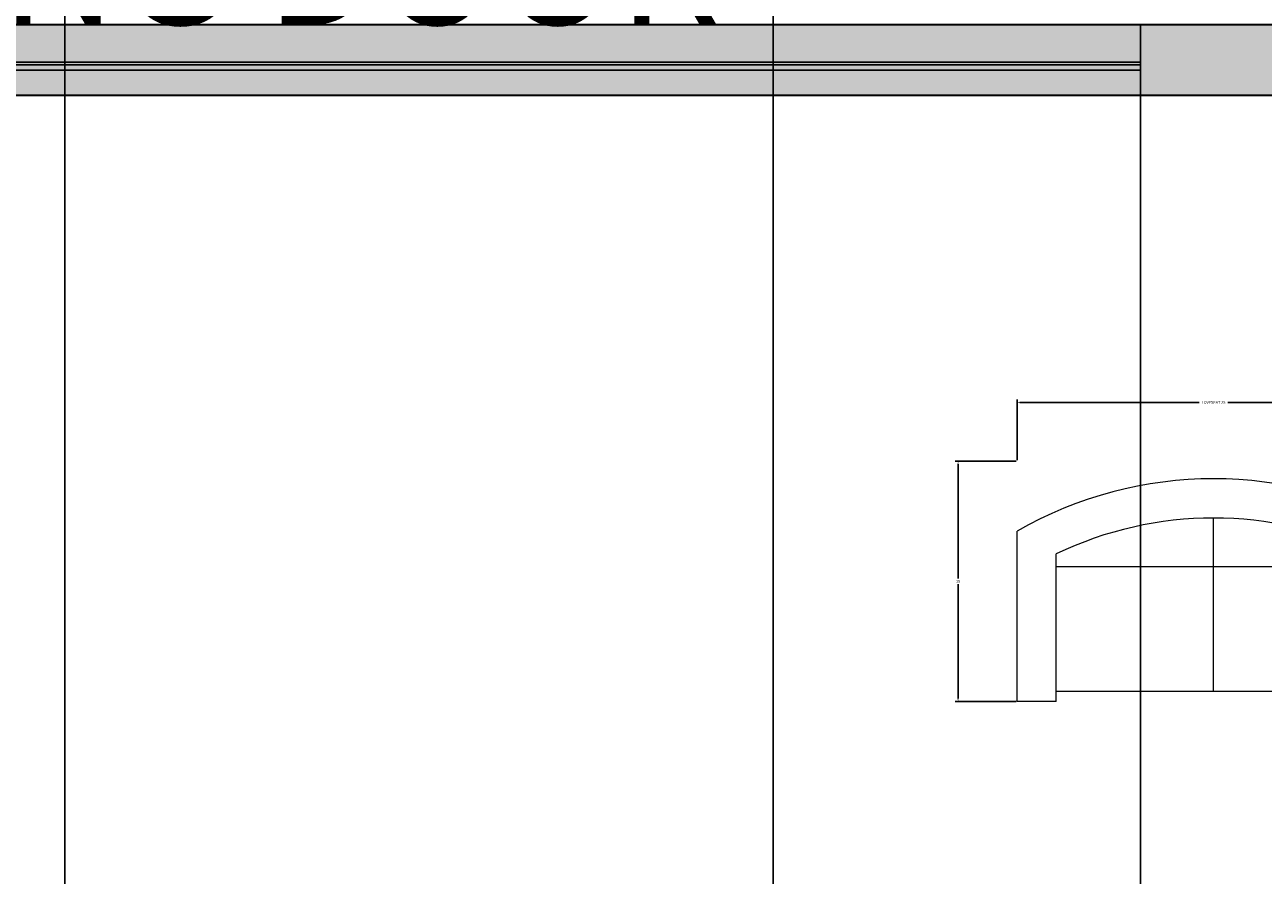
# Model space of a CAD drawing. Units: inches. Extents: x 857 to 1111, y 424 to 822.
# Tile 7 of 9: x 983 to 1062, y 668 to 722. Entities that reach past the tile are written whole.
import ezdxf

# ---------------------------------------------------------------- set-up
doc = ezdxf.new("R2010")
doc.units = ezdxf.units.IN
for name, color, linetype, lineweight in [('A-ANNO-DIMS', 2, 'Continuous', 18), ('A-ANNO-TEXT', 7, 'Continuous', 18), ('A-DOOR', 3, 'Continuous', 25), ('A-DOOR-PATT', 17, 'Continuous', 13), ('A-FURN', 8, 'Continuous', 18), ('A-WALL', 7, 'Continuous', 35), ('A-WALL-PATT', 252, 'Continuous', 13)]:
    doc.layers.add(name, color=color, linetype=linetype, lineweight=lineweight)
doc.styles.get("Standard").update_dxf_attribs({"font": 'arial.ttf'})
doc.dimstyles.get("Standard").update_dxf_attribs({"dimtxt": 0.18, "dimasz": 0.18, "dimexe": 0.18, "dimexo": 0.0625, "dimgap": 0.09, "dimtad": 0, "dimtih": 1, "dimtoh": 1, "dimdec": 4, "dimzin": 0, "dimdsep": 46, "dimtxsty": 'Standard', "dimcen": 0.09, "dimadec": 0, "dimazin": 0, "dimtfac": 1, "dimtdec": 4, "dimtofl": 0, "dimtmove": 0, "dimatfit": 3, "dimfxl": 1, "dimtolj": 1, "dimtzin": 0, "dimarcsym": 0})

# ---------------------------------------------------------------- blocks, each defined once
blk = doc.blocks.new('Sofa - Roundback Loveseat 5 ft.')
for p, q in [((0, -32.44198), (0, -5.99998)), ((-24, -33.99998), (-24, -11.46958)), ((24.00004, -33.99998), (24.00004, -11.46958)), ((-23.9998, -13.38178), (23.99986, -13.38178)), ((-24, -32.44198), (24.00004, -32.44198))]:
    blk.add_line(p, q)
for points in [[(-24, -33.99998), (-30, -33.99998), (-30, -7.99998)], [(30.00004, -7.99998), (30.00004, -33.99998), (24.00004, -33.99998)]]:
    blk.add_lwpolyline(points)
for centre, radius, start, end in [((0, -60.24998), 60.24998, 60.13715, 119.8628), ((0, -61.38438), 55.38444, 64.32083, 115.6792)]:
    blk.add_arc(centre, radius, start, end)
blk = doc.blocks.new('*D36')
at = {"layer": 'A-ANNO-DIMS', "color": 0, "lineweight": -2, "transparency": 16777216}
for p, q in [((1046.13, 694.165), (1046.13, 698.028)), ((1071.104, 694.165), (1071.104, 698.028)), ((1046.31, 697.848), (1057.702, 697.848)), ((1070.924, 697.848), (1059.531, 697.848))]:
    blk.add_line(p, q, dxfattribs=at)
at = {"layer": 'A-ANNO-DIMS', "color": 0, "transparency": 16777216}
for points in [[(1046.31, 697.878), (1046.31, 697.818), (1046.13, 697.848)], [(1070.924, 697.878), (1070.924, 697.818), (1071.104, 697.848)]]:
    blk.add_solid(points, dxfattribs=at)
at = {"layer": 'Defpoints', "color": 0, "transparency": 16777216}
for p in [(1071.104, 697.848), (1046.13, 694.102), (1071.104, 694.102)]:
    blk.add_point(p, dxfattribs=at)
at = {"layer": 'A-ANNO-DIMS', "color": 0, "transparency": 16777216, "insert": (1058.617, 697.848), "char_height": 0.18, "attachment_point": 5}
blk.add_mtext('\\A1;LOVESEAT 25', dxfattribs=at)
blk = doc.blocks.new('*D37')
at = {"layer": 'A-ANNO-DIMS', "color": 0, "lineweight": -2, "transparency": 16777216}
for p, q in [((1046.067, 694.102), (1042.203, 694.102)), ((1042.383, 693.922), (1042.383, 686.653)), ((1042.383, 679.02), (1042.383, 686.289)), ((1046.067, 678.84), (1042.203, 678.84))]:
    blk.add_line(p, q, dxfattribs=at)
at = {"layer": 'A-ANNO-DIMS', "color": 0, "transparency": 16777216}
for points in [[(1042.353, 693.922), (1042.413, 693.922), (1042.383, 694.102)], [(1042.353, 679.02), (1042.413, 679.02), (1042.383, 678.84)]]:
    blk.add_solid(points, dxfattribs=at)
at = {"layer": 'Defpoints', "color": 0, "transparency": 16777216}
for p in [(1042.383, 694.102), (1046.13, 694.102), (1046.13, 678.84)]:
    blk.add_point(p, dxfattribs=at)
at = {"layer": 'A-ANNO-DIMS', "color": 0, "transparency": 16777216, "insert": (1042.383, 686.471), "char_height": 0.18, "attachment_point": 5}
blk.add_mtext('\\A1;15', dxfattribs=at)
blk = doc.blocks.new('*D48')
at = {"layer": 'A-ANNO-DIMS', "color": 0, "lineweight": -2, "transparency": 16777216}
for p, q in [((885.137, 582.419), (885.137, 822.087)), ((885.317, 821.907), (935.001, 821.907)), ((985.457, 821.907), (935.773, 821.907)), ((985.637, 582.419), (985.637, 822.087))]:
    blk.add_line(p, q, dxfattribs=at)
at = {"layer": 'A-ANNO-DIMS', "color": 0, "transparency": 16777216}
for points in [[(885.317, 821.937), (885.317, 821.877), (885.137, 821.907)], [(985.457, 821.937), (985.457, 821.877), (985.637, 821.907)]]:
    blk.add_solid(points, dxfattribs=at)
at = {"layer": 'Defpoints', "color": 0, "transparency": 16777216}
for p in [(985.637, 821.907), (885.137, 582.357), (985.637, 582.357)]:
    blk.add_point(p, dxfattribs=at)
at = {"layer": 'A-ANNO-DIMS', "color": 0, "transparency": 16777216, "insert": (935.387, 821.907), "char_height": 0.18, "attachment_point": 5}
blk.add_mtext('\\A1;100.5', dxfattribs=at)
blk = doc.blocks.new('*D49')
at = {"layer": 'A-ANNO-DIMS', "color": 0, "lineweight": -2, "transparency": 16777216}
for p, q in [((985.637, 451.919), (985.637, 822.087)), ((985.817, 821.907), (1007.914, 821.907)), ((1030.457, 821.907), (1008.36, 821.907)), ((1030.637, 451.919), (1030.637, 822.087))]:
    blk.add_line(p, q, dxfattribs=at)
at = {"layer": 'A-ANNO-DIMS', "color": 0, "transparency": 16777216}
for points in [[(985.817, 821.937), (985.817, 821.877), (985.637, 821.907)], [(1030.457, 821.937), (1030.457, 821.877), (1030.637, 821.907)]]:
    blk.add_solid(points, dxfattribs=at)
at = {"layer": 'Defpoints', "color": 0, "transparency": 16777216}
for p in [(1030.637, 821.907), (985.637, 451.857), (1030.637, 451.857)]:
    blk.add_point(p, dxfattribs=at)
at = {"layer": 'A-ANNO-DIMS', "color": 0, "transparency": 16777216, "insert": (1008.137, 821.907), "char_height": 0.18, "attachment_point": 5}
blk.add_mtext('\\A1;45', dxfattribs=at)
blk = doc.blocks.new('*D55')
at = {"layer": 'A-ANNO-DIMS', "color": 0, "lineweight": -2, "transparency": 16777216}
for p, q in [((1053.972, 717.294), (1053.972, 423.627)), ((1083.137, 717.294), (1083.137, 423.627)), ((1054.152, 423.807), (1068.088, 423.807)), ((1082.957, 423.807), (1069.02, 423.807))]:
    blk.add_line(p, q, dxfattribs=at)
at = {"layer": 'A-ANNO-DIMS', "color": 0, "transparency": 16777216}
for points in [[(1054.152, 423.837), (1054.152, 423.777), (1053.972, 423.807)], [(1082.957, 423.837), (1082.957, 423.777), (1083.137, 423.807)]]:
    blk.add_solid(points, dxfattribs=at)
at = {"layer": 'Defpoints', "color": 0, "transparency": 16777216}
for p in [(1053.972, 717.357), (1083.137, 717.357), (1083.137, 423.807)]:
    blk.add_point(p, dxfattribs=at)
at = {"layer": 'A-ANNO-DIMS', "color": 0, "transparency": 16777216, "insert": (1068.554, 423.807), "char_height": 0.18, "attachment_point": 5}
blk.add_mtext('\\A1;29.165', dxfattribs=at)
blk = doc.blocks.new('*D56')
at = {"layer": 'A-ANNO-DIMS', "color": 0, "lineweight": -2, "transparency": 16777216}
for p, q in [((924.77, 717.294), (924.77, 423.627)), ((1053.972, 717.294), (1053.972, 423.627)), ((924.95, 423.807), (988.986, 423.807)), ((1053.792, 423.807), (989.755, 423.807))]:
    blk.add_line(p, q, dxfattribs=at)
at = {"layer": 'A-ANNO-DIMS', "color": 0, "transparency": 16777216}
for points in [[(924.95, 423.837), (924.95, 423.777), (924.77, 423.807)], [(1053.792, 423.837), (1053.792, 423.777), (1053.972, 423.807)]]:
    blk.add_solid(points, dxfattribs=at)
at = {"layer": 'Defpoints', "color": 0, "transparency": 16777216}
for p in [(924.77, 717.357), (1053.972, 717.357), (1053.972, 423.807)]:
    blk.add_point(p, dxfattribs=at)
at = {"layer": 'A-ANNO-DIMS', "color": 0, "transparency": 16777216, "insert": (989.371, 423.807), "char_height": 0.18, "attachment_point": 5}
blk.add_mtext('\\A1;129.2', dxfattribs=at)

msp = doc.modelspace()

# ---------------------------------------------------------------- hatches: boundary and pattern name
at = {"layer": 'A-DOOR-PATT'}
h = msp.add_hatch(color=256, dxfattribs=at)
h.dxf.hatch_style = 1
h.set_gradient(color1=(0, 0, 255), color2=(255, 255, 0))
h.paths.add_polyline_path([(1053.9717, 718.9594), (969.1676, 718.9594), (969.1596, 718.4668), (927.0274, 718.4668), (924.7696, 718.4668), (924.7696, 717.3567), (1053.9717, 717.3567)], flags=17)
h.paths.add_polyline_path([(969.1676, 718.9594), (969.1922, 720.4869), (927.0274, 720.4869, -0.9340935), (927.0274, 718.4668), (969.1596, 718.4668)], flags=0)
h.paths.add_polyline_path([(1053.9717, 721.8567), (924.7696, 721.8567), (924.7696, 720.4869), (926.8896, 720.4869, -0.0340762), (927.0274, 720.4869), (927.0302, 720.4869), (969.1922, 720.4869), (969.1759, 719.4769), (1053.9717, 719.4769)], flags=17)
h.paths.add_polyline_path([(1053.9717, 721.8567), (924.7696, 721.8567), (924.7696, 717.3567), (1053.9717, 717.3567)])
h.paths.add_polyline_path([(969.1596, 718.4668), (927.0274, 718.4668, 0.9340935), (927.0274, 720.4869), (969.1922, 720.4869)], flags=16)
h = msp.add_hatch(color=256, dxfattribs=at)
h.dxf.hatch_style = 1
h.set_gradient(color1=(0, 0, 255), color2=(255, 255, 0), name='INVCYLINDER')
h.paths.add_polyline_path([(1053.9717, 721.8567), (924.7696, 721.8567), (924.7696, 720.4869), (927.0302, 720.4869), (969.1922, 720.4869), (969.1759, 719.4769), (1053.9717, 719.4769)], flags=17)
h.paths.add_polyline_path([(1053.9717, 718.9594), (969.1676, 718.9594), (969.1759, 719.4769), (1053.9717, 719.4769), (1053.9717, 721.8567), (924.7696, 721.8567), (924.7696, 717.3567), (1053.9717, 717.3567)])
h.paths.add_polyline_path([(969.1596, 718.4668), (927.0274, 718.4668, 0.9340935), (927.0274, 720.4869), (969.1922, 720.4869)], flags=16)
h = msp.add_hatch(color=256, dxfattribs=at)
h.dxf.hatch_style = 1
h.set_gradient(color1=(0, 0, 255), color2=(255, 255, 0), name='SPHERICAL')
h.paths.add_polyline_path([(1053.9717, 721.8567), (924.7696, 721.8567), (924.7696, 717.3567), (1053.9717, 717.3567), (1053.9717, 718.9594), (969.1676, 718.9594), (969.1759, 719.4769), (1053.9717, 719.4769)])
h.paths.add_polyline_path([(927.0274, 720.4869, -0.9340935), (927.0274, 718.4668), (969.1596, 718.4668), (969.1922, 720.4869)], flags=16)
at = {"layer": 'A-WALL-PATT'}
h = msp.add_hatch(color=256, dxfattribs=at)
h.dxf.hatch_style = 1
h.paths.add_polyline_path([(924.7696, 721.8567), (885.1369, 721.8567), (885.1369, 793.8567), (1083.1369, 793.8567), (1083.1369, 721.8567), (1053.9717, 721.8567), (1053.9717, 717.3567), (1083.1369, 717.3567), (1083.1369, 706.6069), (1092.1369, 706.6069), (1092.1369, 802.8567), (876.1369, 802.8567), (876.1369, 664.6868), (885.1369, 664.6868), (885.1369, 717.3567), (924.7696, 717.3567)])
h.paths.add_polyline_path([(985.6369, 582.3567), (885.1369, 582.3567), (885.1369, 585.1154), (885.1369, 628.6868), (876.1369, 628.6868), (876.1369, 529.0363), (885.1369, 529.0363), (885.1369, 577.8567), (981.1369, 577.8567), (985.6369, 577.8567)])
h.paths.add_polyline_path([(885.1369, 493.0363), (876.1369, 493.0363), (876.1369, 442.8567), (991.6369, 442.8567), (991.6369, 451.8567), (985.6369, 451.8567), (985.6369, 535.8567), (981.1369, 535.8567), (981.1369, 451.8567), (885.1369, 451.8567)])
h.paths.add_polyline_path([(1092.1369, 553.8025), (1083.1369, 553.8025), (1083.1369, 451.8567), (1030.6369, 451.8567), (1027.6369, 451.8567), (1027.6369, 442.8567), (1092.1369, 442.8567)])
h.paths.add_polyline_path([(1092.1369, 670.6069), (1083.1369, 670.6069), (1083.1369, 662.5384, -0.0267686), (1083.1369, 657.4501), (1083.1369, 589.8025), (1092.1369, 589.8025)])

# ---------------------------------------------------------------- linework, layer by layer
at = {"layer": 'A-DOOR'}
for p, q in [((969.1734, 719.3176), (1053.9717, 719.3176)), ((969.1759, 719.4769), (1053.9717, 719.4769)), ((969.1676, 718.9594), (1053.9717, 718.9594))]:
    msp.add_line(p, q, dxfattribs=at)
msp.add_lwpolyline([(924.7696, 721.8567), (1053.9717, 721.8567), (1053.9717, 717.3567), (924.7696, 717.3567)], close=True, dxfattribs=at)
at = {"layer": 'A-WALL'}
for p, q in [((1083.1369, 721.8567), (885.1369, 721.8567)), ((1083.1369, 717.3567), (885.1369, 717.3567))]:
    msp.add_line(p, q, dxfattribs=at)

# ---------------------------------------------------------------- block references
at = {"layer": 'A-FURN', "xscale": 0.416233368792988, "yscale": 0.416233368792988, "zscale": 0.416233368792988}
msp.add_blockref('Sofa - Roundback Loveseat 5 ft.', (1058.6165, 692.9922), dxfattribs=at)

# ---------------------------------------------------------------- texts
at = {"layer": 'A-ANNO-TEXT'}
msp.add_text('SLIDING DOOR ', height=7.55928, dxfattribs=at).set_placement((956.6211, 721.8567))

# ---------------------------------------------------------------- dimensions: what is measured, and where the dimension line sits
at = {"layer": 'A-ANNO-DIMS'}
for base, p1, p2, override, picture, middle in [((985.6369, 821.9067), (885.1369, 582.3567), (985.6369, 582.3567), {"dimdec": 1, "dimlfac": 1, "dimrnd": 0, "dimzin": 0, "dimdsep": 46, "dimlunit": 2}, '*D48', (935.3869, 821.9067)), ((1030.6369, 821.9067), (985.6369, 451.8567), (1030.6369, 451.8567), {"dimdec": 0, "dimlfac": 1, "dimrnd": 0, "dimzin": 0, "dimdsep": 46, "dimlunit": 2}, '*D49', (1008.1369, 821.9067)), ((1053.9717, 423.8067), (924.7696, 717.3567), (1053.9717, 717.3567), {"dimdec": 1, "dimlfac": 1, "dimrnd": 0, "dimzin": 0, "dimdsep": 46, "dimlunit": 2}, '*D56', (989.3707, 423.8067)), ((1083.1369, 423.8067), (1053.9717, 717.3567), (1083.1369, 717.3567), {"dimdec": 3, "dimlfac": 1, "dimrnd": 0, "dimzin": 0, "dimdsep": 46, "dimlunit": 2}, '*D55', (1068.5543, 423.8067))]:
    dim = msp.add_linear_dim(base=base, p1=p1, p2=p2, dimstyle='Standard', override=override, dxfattribs=at)
    dim.commit()
    dim.dimension.update_dxf_attribs({"geometry": picture, "text_midpoint": middle})
dim = msp.add_linear_dim(base=(1071.1035, 697.8482), p1=(1046.1295, 694.1021), p2=(1071.1035, 694.1021), text='LOVESEAT <>', dimstyle='Standard', override={"dimdec": 0, "dimlfac": 1, "dimrnd": 0, "dimzin": 0, "dimdsep": 46, "dimlunit": 2}, dxfattribs=at)
dim.commit()
dim.dimension.update_dxf_attribs({"geometry": '*D36', "text_midpoint": (1058.6165, 697.8482)})
dim = msp.add_linear_dim(base=(1042.3834, 694.1021), p1=(1046.1295, 678.8402), p2=(1046.1295, 694.1021), angle=90, dimstyle='Standard', override={"dimdec": 0, "dimlfac": 1, "dimrnd": 0, "dimzin": 0, "dimdsep": 46, "dimlunit": 2}, dxfattribs=at)
dim.commit()
dim.dimension.update_dxf_attribs({"geometry": '*D37', "text_midpoint": (1042.3834, 686.4712)})

doc.saveas('drawing.dxf')
